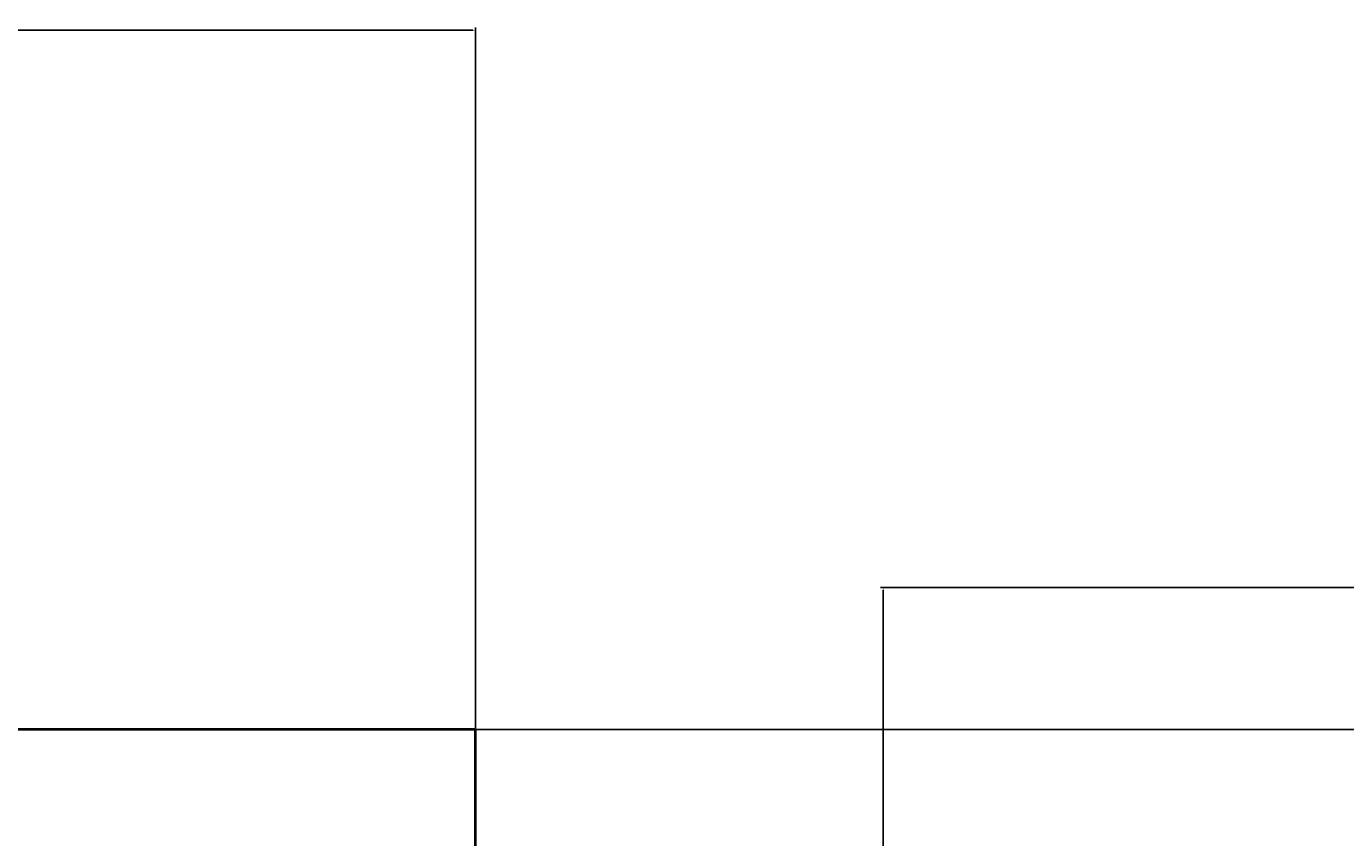
# Model space of a CAD drawing. Units: inches. Extents: x -301 to 715, y -607 to 364.
# Tile 125 of 141: x 101 to 194, y 303 to 360. Entities that reach past the tile are written whole.
import ezdxf

# ---------------------------------------------------------------- set-up
doc = ezdxf.new("R2010")
doc.units = ezdxf.units.IN
doc.header["$MEASUREMENT"] = 0
doc.layers.add('A-ANNO-DIMS', color=2, linetype='Continuous', lineweight=18)
doc.layers.add('A-WALL', color=3, linetype='Continuous', lineweight=40)
doc.styles.get("Standard").update_dxf_attribs({"font": 'arial.ttf'})
doc.dimstyles.get("Standard").update_dxf_attribs({"dimtxt": 0.18, "dimasz": 0.18, "dimexe": 0.18, "dimexo": 0.0625, "dimgap": 0.09, "dimtad": 0, "dimtih": 1, "dimtoh": 1, "dimdec": 1, "dimzin": 0, "dimdsep": 46, "dimlunit": 4, "dimtxsty": 'Standard', "dimcen": 0.09, "dimclrd": 3, "dimclre": 4, "dimclrt": 6, "dimadec": 0, "dimazin": 0, "dimtfac": 1, "dimtdec": 1, "dimtofl": 0, "dimtmove": 0, "dimatfit": 3, "dimfxl": 1, "dimtfill": 2, "dimtfillclr": 51, "dimtolj": 1, "dimtzin": 0, "dimarcsym": 0})

# ---------------------------------------------------------------- blocks, each defined once
blk = doc.blocks.new('*D144')
at = {"layer": 'A-ANNO-DIMS', "color": 4, "lineweight": -2, "transparency": 16777216}
for p, q in [((-204.603, 310.245), (-204.603, 359.612)), ((132.897, 310.245), (132.897, 359.612))]:
    blk.add_line(p, q, dxfattribs=at)
at = {"layer": 'A-ANNO-DIMS', "color": 3, "lineweight": -2, "transparency": 16777216}
for p, q in [((-204.423, 359.432), (-36.464, 359.432)), ((132.717, 359.432), (-35.243, 359.432))]:
    blk.add_line(p, q, dxfattribs=at)
at = {"layer": 'A-ANNO-DIMS', "color": 3, "transparency": 16777216}
for points in [[(-204.423, 359.462), (-204.423, 359.402), (-204.603, 359.432)], [(132.717, 359.462), (132.717, 359.402), (132.897, 359.432)]]:
    blk.add_solid(points, dxfattribs=at)
at = {"layer": 'Defpoints', "color": 0, "transparency": 16777216}
for p in [(132.897, 359.432), (-204.603, 310.182), (132.897, 310.182)]:
    blk.add_point(p, dxfattribs=at)
at = {"layer": 'A-ANNO-DIMS', "color": 6, "transparency": 16777216, "insert": (-35.853, 359.432), "char_height": 0.18, "attachment_point": 5, "bg_fill": 1, "box_fill_scale": 1.25, "bg_fill_color": 51, "bg_fill_transparency": 0}
blk.add_mtext('\\A1;28\'-1 1/2"', dxfattribs=at)
blk = doc.blocks.new('*D153')
at = {"layer": 'A-ANNO-DIMS', "color": 4, "lineweight": -2, "transparency": 16777216}
for p, q in [((132.959, 310.182), (233.659, 310.182)), ((123.959, 193.182), (233.659, 193.182))]:
    blk.add_line(p, q, dxfattribs=at)
at = {"layer": 'A-ANNO-DIMS', "color": 3, "lineweight": -2, "transparency": 16777216}
for p, q in [((233.479, 310.002), (233.479, 251.864)), ((233.479, 193.362), (233.479, 251.5))]:
    blk.add_line(p, q, dxfattribs=at)
at = {"layer": 'A-ANNO-DIMS', "color": 3, "transparency": 16777216}
for points in [[(233.449, 310.002), (233.509, 310.002), (233.479, 310.182)], [(233.449, 193.362), (233.509, 193.362), (233.479, 193.182)]]:
    blk.add_solid(points, dxfattribs=at)
at = {"layer": 'Defpoints', "color": 0, "transparency": 16777216}
for p in [(132.897, 310.182), (123.897, 193.182), (233.479, 193.182)]:
    blk.add_point(p, dxfattribs=at)
at = {"layer": 'A-ANNO-DIMS', "color": 6, "transparency": 16777216, "insert": (233.479, 251.682), "char_height": 0.18, "attachment_point": 5, "bg_fill": 1, "box_fill_scale": 1.25, "bg_fill_color": 51, "bg_fill_transparency": 0}
blk.add_mtext('\\A1;9\'-9"', dxfattribs=at)
blk = doc.blocks.new('*D154')
at = {"layer": 'A-ANNO-DIMS', "color": 4, "lineweight": -2, "transparency": 16777216}
for p, q in [((9.897, 310.245), (9.897, 359.612)), ((132.897, 310.245), (132.897, 359.612))]:
    blk.add_line(p, q, dxfattribs=at)
at = {"layer": 'A-ANNO-DIMS', "color": 3, "lineweight": -2, "transparency": 16777216}
for p, q in [((10.077, 359.432), (71.006, 359.432)), ((132.717, 359.432), (71.787, 359.432))]:
    blk.add_line(p, q, dxfattribs=at)
at = {"layer": 'A-ANNO-DIMS', "color": 3, "transparency": 16777216}
for points in [[(10.077, 359.462), (10.077, 359.402), (9.897, 359.432)], [(132.717, 359.462), (132.717, 359.402), (132.897, 359.432)]]:
    blk.add_solid(points, dxfattribs=at)
at = {"layer": 'Defpoints', "color": 0, "transparency": 16777216}
for p in [(132.897, 359.432), (9.897, 310.182), (132.897, 310.182)]:
    blk.add_point(p, dxfattribs=at)
at = {"layer": 'A-ANNO-DIMS', "color": 6, "transparency": 16777216, "insert": (71.397, 359.432), "char_height": 0.18, "attachment_point": 5, "bg_fill": 1, "box_fill_scale": 1.25, "bg_fill_color": 51, "bg_fill_transparency": 0}
blk.add_mtext('\\A1;10\'-3"', dxfattribs=at)
blk = doc.blocks.new('*D162')
at = {"layer": 'A-ANNO-DIMS', "color": 4, "lineweight": -2, "transparency": 16777216}
for p, q in [((222.328, 320.182), (161.439, 320.182)), ((222.328, -233.818), (161.439, -233.818))]:
    blk.add_line(p, q, dxfattribs=at)
at = {"layer": 'A-ANNO-DIMS', "color": 3, "lineweight": -2, "transparency": 16777216}
for p, q in [((161.619, 320.002), (161.619, 43.364)), ((161.619, -233.638), (161.619, 43))]:
    blk.add_line(p, q, dxfattribs=at)
at = {"layer": 'A-ANNO-DIMS', "color": 3, "transparency": 16777216}
for points in [[(161.589, 320.002), (161.649, 320.002), (161.619, 320.182)], [(161.589, -233.638), (161.649, -233.638), (161.619, -233.818)]]:
    blk.add_solid(points, dxfattribs=at)
at = {"layer": 'Defpoints', "color": 0, "transparency": 16777216}
for p in [(161.619, 320.182), (222.39, 320.182), (222.39, -233.818)]:
    blk.add_point(p, dxfattribs=at)
at = {"layer": 'A-ANNO-DIMS', "color": 6, "transparency": 16777216, "insert": (161.619, 43.182), "char_height": 0.18, "attachment_point": 5, "bg_fill": 1, "box_fill_scale": 1.25, "bg_fill_color": 51, "bg_fill_transparency": 0}
blk.add_mtext('\\A1;46\'-2"', dxfattribs=at)

msp = doc.modelspace()

# ---------------------------------------------------------------- linework, layer by layer
at = {"layer": 'A-WALL'}
for p, q in [((132.897, 310.182), (-204.603, 310.182)), ((132.897, 199.182), (132.897, 310.182))]:
    msp.add_line(p, q, dxfattribs=at)

# ---------------------------------------------------------------- dimensions: what is measured, and where the dimension line sits
at = {"layer": 'A-ANNO-DIMS'}
for p1, picture, middle in [((-204.603, 310.182), '*D144', (-35.853, 359.432)), ((9.897, 310.182), '*D154', (71.397, 359.432))]:
    dim = msp.add_linear_dim(base=(132.897, 359.432), p1=p1, p2=(132.897, 310.182), dimstyle='Standard', override={"dimdec": 1, "dimlfac": 1, "dimrnd": 0, "dimzin": 1, "dimdsep": 46, "dimlunit": 4, "dimfrac": 2}, dxfattribs=at)
    dim.commit()
    dim.dimension.update_dxf_attribs({"geometry": picture, "text_midpoint": middle})
for base, p1, p2, picture, middle in [((161.619, 320.182), (222.39, -233.818), (222.39, 320.182), '*D162', (161.619, 43.182)), ((233.479, 193.182), (132.897, 310.182), (123.897, 193.182), '*D153', (233.479, 251.682))]:
    dim = msp.add_linear_dim(base=base, p1=p1, p2=p2, angle=90, dimstyle='Standard', override={"dimdec": 1, "dimlfac": 1, "dimrnd": 0, "dimzin": 1, "dimdsep": 46, "dimlunit": 4, "dimfrac": 2}, dxfattribs=at)
    dim.commit()
    dim.dimension.update_dxf_attribs({"geometry": picture, "text_midpoint": middle})

doc.saveas('drawing.dxf')
